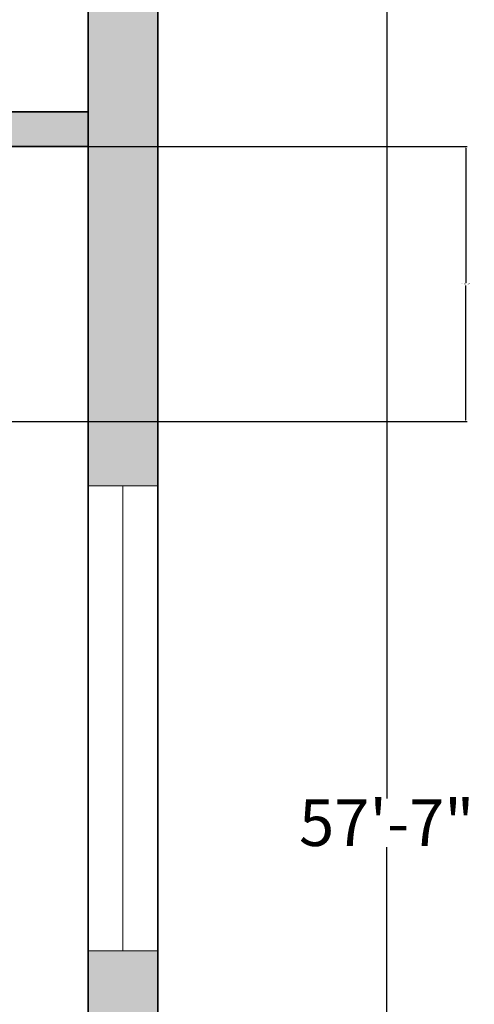
# Model space of a CAD drawing. Units: inches. Extents: x -15 to 423, y -713 to 71.
# Tile 17 of 24: x 364 to 423, y -351 to -224. Entities that reach past the tile are written whole.
import ezdxf

# ---------------------------------------------------------------- set-up
doc = ezdxf.new("R2010")
doc.units = ezdxf.units.IN
doc.header["$MEASUREMENT"] = 0
for name, color, linetype, lineweight in [('A-ANNO-DIMS', 2, 'Continuous', 18), ('A-GLAZ', 5, 'Continuous', 18), ('A-WALL', 7, 'Continuous', 35), ('A-WALL-PATT', 8, 'Continuous', 13)]:
    doc.layers.add(name, color=color, linetype=linetype, lineweight=lineweight)
doc.styles.get("Standard").update_dxf_attribs({"font": 'arial.ttf'})
doc.dimstyles.get("Standard").update_dxf_attribs({"dimtxt": 0.18, "dimasz": 0.18, "dimexe": 0.18, "dimexo": 0.0625, "dimgap": 0.09, "dimtad": 0, "dimtih": 1, "dimtoh": 1, "dimdec": 0, "dimzin": 0, "dimdsep": 46, "dimlunit": 3, "dimtxsty": 'Standard', "dimcen": 0.09, "dimadec": 0, "dimazin": 0, "dimtfac": 1, "dimtdec": 0, "dimtofl": 0, "dimtmove": 0, "dimatfit": 3, "dimfxl": 1, "dimtolj": 1, "dimtzin": 0, "dimarcsym": 0})

# ---------------------------------------------------------------- blocks, each defined once
blk = doc.blocks.new('*D9')
at = {"layer": 'A-ANNO-DIMS', "color": 0, "lineweight": -2, "transparency": 16777216}
for p, q in [((382.14, 17.5), (411.79, 17.5)), ((411.61, 17.32), (411.61, -324.61)), ((411.61, -672.82), (411.61, -330.89)), ((382.14, -673), (411.79, -673))]:
    blk.add_line(p, q, dxfattribs=at)
at = {"layer": 'A-ANNO-DIMS', "color": 0, "transparency": 16777216}
for points in [[(411.58, 17.32), (411.64, 17.32), (411.61, 17.5)], [(411.58, -672.82), (411.64, -672.82), (411.61, -673)]]:
    blk.add_solid(points, dxfattribs=at)
at = {"layer": 'Defpoints', "color": 0, "transparency": 16777216}
for p in [(382.08, 17.5), (382.08, -673), (411.61, -673)]:
    blk.add_point(p, dxfattribs=at)
at = {"layer": 'A-ANNO-DIMS', "color": 0, "transparency": 16777216, "insert": (411.61, -327.75), "char_height": 6, "attachment_point": 5}
blk.add_mtext('\\A1;57\'-7"', dxfattribs=at)
blk = doc.blocks.new('WINDOW-60IN')
for p, q in [((0, 9), (60, 9)), ((0, 0), (0, 9)), ((60, 9), (60, 0)), ((0, 4.5), (60, 4.5)), ((60, 0), (0, 0))]:
    blk.add_line(p, q)
blk = doc.blocks.new('*D38')
at = {"layer": 'A-ANNO-DIMS', "color": 0, "lineweight": -2, "transparency": 16777216}
for p, q in [((124.14, -240.5), (422.01, -240.5)), ((421.83, -240.68), (421.83, -258.06)), ((421.83, -275.8), (421.83, -258.42)), ((124.14, -275.98), (422.01, -275.98))]:
    blk.add_line(p, q, dxfattribs=at)
at = {"layer": 'A-ANNO-DIMS', "color": 0, "transparency": 16777216}
for points in [[(421.8, -240.68), (421.86, -240.68), (421.83, -240.5)], [(421.8, -275.8), (421.86, -275.8), (421.83, -275.98)]]:
    blk.add_solid(points, dxfattribs=at)
at = {"layer": 'Defpoints', "color": 0, "transparency": 16777216}
for p in [(124.08, -240.5), (124.08, -275.98), (421.83, -275.98)]:
    blk.add_point(p, dxfattribs=at)
at = {"layer": 'A-ANNO-DIMS', "color": 0, "transparency": 16777216, "insert": (421.83, -258.24), "char_height": 0.18, "attachment_point": 5}
blk.add_mtext('\\A1;2\'-11 1/2"', dxfattribs=at)

msp = doc.modelspace()

# ---------------------------------------------------------------- hatches: boundary and pattern name
at = {"layer": 'A-WALL-PATT'}
h = msp.add_hatch(color=256, dxfattribs=at)
h.dxf.hatch_style = 1
h.paths.add_polyline_path([(34.08, -349.58), (25.08, -349.58), (25.08, -431), (34.08, -431)])
h.paths.add_polyline_path([(34.08, -467), (25.08, -467), (25.08, -673), (34.08, -673)])
h.paths.add_polyline_path([(373.08, -668.5), (182.08, -668.5), (182.08, -673), (373.08, -673)])
h.paths.add_polyline_path([(253.2, -597.5), (191.08, -597.5), (191.08, -594.5), (182.08, -594.5), (182.08, -606.5), (253.2, -606.5)])
h.paths.add_polyline_path([(373.08, -597.5), (313.2, -597.5), (313.2, -606.5), (373.08, -606.5)])
h.paths.add_polyline_path([(382.08, -545.55), (373.08, -545.55), (373.08, -673), (382.08, -673)])
h.paths.add_polyline_path([(139.08, -488), (34.08, -488), (34.08, -497), (139.08, -497), (139.08, -492.5)])
h.paths.add_polyline_path([(139.08, -396.5), (128.58, -396.5), (128.58, -352.79), (124.08, -352.79), (124.08, -396.5), (34.08, -396.5), (34.08, -410), (139.08, -410), (139.08, -403.25)])
h.paths.add_polyline_path([(191.08, -396.5), (179.08, -396.5), (179.08, -410), (182.08, -410), (182.08, -488), (179.08, -488), (179.08, -497), (182.08, -497), (182.08, -501.43), (191.08, -501.43)])
h.paths.add_polyline_path([(373.08, -396.5), (253.08, -396.5), (253.08, -393.5), (248.58, -393.5), (248.58, -401), (284.58, -401), (284.58, -404), (289.08, -404), (289.08, -401), (373.08, -401)])
h.paths.add_polyline_path([(373.08, -449), (289.08, -449), (289.08, -432), (286.83, -432), (284.58, -432), (284.58, -453.5), (373.08, -453.5)])
h.paths.add_polyline_path([(382.08, -344.27), (373.08, -344.27), (373.08, -413.68), (382.08, -413.68)])
h.paths.add_polyline_path([(382.08, -437.68), (373.08, -437.68), (373.08, -485.55), (382.08, -485.55)])
h.paths.add_polyline_path([(34.08, -188.26), (25.08, -188.26), (25.08, -289.58), (34.08, -289.58)])
h.paths.add_polyline_path([(164.08, -236), (34.08, -236), (34.08, -240.5), (124.08, -240.5), (124.08, -293.12), (128.58, -293.12), (128.58, -240.5), (164.08, -240.5), (164.08, -238.25)])
h.paths.add_polyline_path([(373.08, -236), (242.58, -236), (242.58, -238.25), (242.58, -240.5), (248.58, -240.5), (248.58, -353.5), (250.83, -353.5), (253.08, -353.5), (253.08, -240.5), (373.08, -240.5)])
h.paths.add_polyline_path([(382.08, -190.86), (373.08, -190.86), (373.08, -284.27), (382.08, -284.27)])
h.paths.add_polyline_path([(211.58, -80), (253.58, -80), (253.58, -77.75), (253.58, -75.5), (153.58, -75.5), (153.58, -77.75), (153.58, -80), (207.08, -80), (207.08, -236), (204.08, -236), (204.08, -240.5), (214.58, -240.5), (214.58, -236), (211.58, -236)])
h.paths.add_polyline_path([(34.08, 8.5), (70.36, 8.5), (70.36, 17.5), (25.08, 17.5), (25.08, -128.26), (34.08, -128.26)])
h.paths.add_polyline_path([(110.58, 17.5), (94.36, 17.5), (94.36, 8.5), (110.58, 8.5)])
h.paths.add_polyline_path([(296.58, 17.5), (110.58, 17.5), (110.58, 13), (296.58, 13)])
h.paths.add_polyline_path([(110.58, 8.5), (106.08, 8.5), (106.08, -75.5), (103.08, -75.5), (103.08, -80), (113.58, -80), (113.58, -77.75), (113.58, -75.5), (110.58, -75.5)])
h.paths.add_polyline_path([(75.08, -75.5), (34.08, -75.5), (34.08, -80), (75.08, -80), (75.08, -77.75)])
h.paths.add_polyline_path([(343.09, 17.5), (296.58, 17.5), (296.58, 13), (296.58, 8.5), (343.09, 8.5)])
h.paths.add_polyline_path([(304.08, -75.5), (301.08, -75.5), (301.08, 8.5), (296.58, 8.5), (296.58, -75.5), (293.58, -75.5), (293.58, -80), (304.08, -80)])
h.paths.add_polyline_path([(382.08, 17.5), (367.09, 17.5), (367.09, 8.5), (373.08, 8.5), (373.08, -130.86), (382.08, -130.86)])
h.paths.add_polyline_path([(373.08, -75.5), (332.08, -75.5), (332.08, -77.75), (332.08, -80), (373.08, -80)])

# ---------------------------------------------------------------- linework, layer by layer
at = {"layer": 'A-WALL'}
for p, q in [((382.08, 17.5), (382.08, -673)), ((373.08, 8.5), (373.08, -673)), ((242.58, -236), (373.08, -236)), ((253.08, -240.5), (373.08, -240.5))]:
    msp.add_line(p, q, dxfattribs=at)

# ---------------------------------------------------------------- block references
at = {"layer": 'A-GLAZ', "rotation": 90.00000000000011}
msp.add_blockref('WINDOW-60IN', (382.08, -344.27), dxfattribs=at)

# ---------------------------------------------------------------- dimensions: what is measured, and where the dimension line sits
at = {"layer": 'A-ANNO-DIMS'}
for base, p1, p2, override, picture, middle in [((411.6050599, -672.99989936), (382.08055573, 17.50010064), (382.08055573, -672.99989936), {"dimtxt": 6, "dimclrd": 0, "dimclre": 0, "dimclrt": 0}, '*D9', (411.6050599, -327.74989936)), ((421.83, -275.98), (124.08, -240.5), (124.08, -275.98), {"dimdec": 1, "dimlfac": 1, "dimrnd": 0, "dimzin": 1, "dimdsep": 46, "dimlunit": 4, "dimfrac": 2}, '*D38', (421.83, -258.24))]:
    dim = msp.add_linear_dim(base=base, p1=p1, p2=p2, angle=90, dimstyle='Standard', override=override, dxfattribs=at)
    dim.commit()
    dim.dimension.update_dxf_attribs({"geometry": picture, "text_midpoint": middle})

doc.saveas('drawing.dxf')
